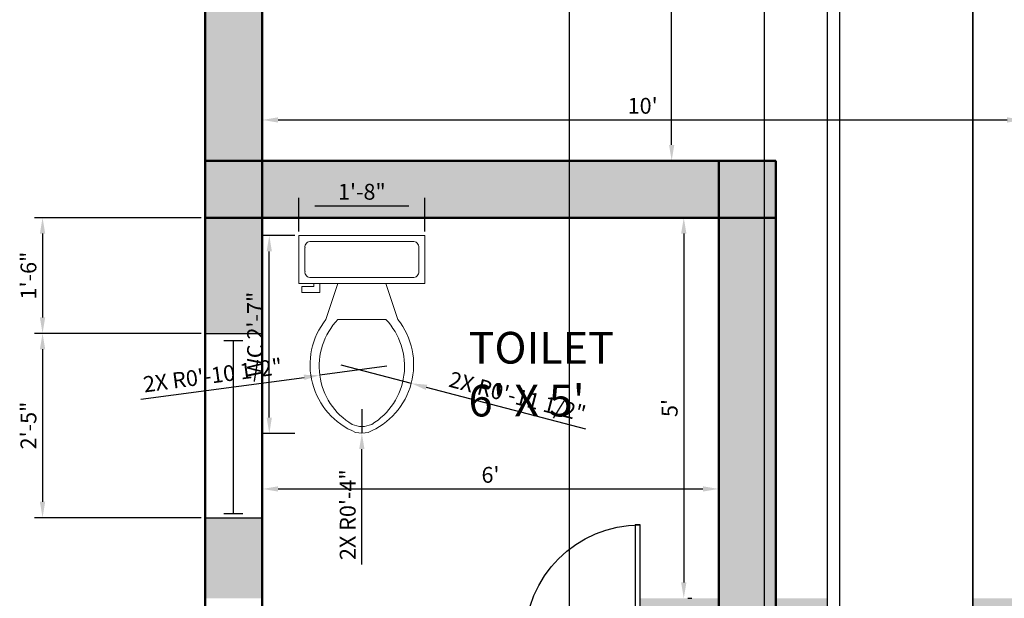
# Model space of a CAD drawing. Units: millimetres. Extents: x 2877 to 3173, y 802 to 1374.
# Tile 3 of 5: x 2879 to 3035, y 1144 to 1236. Entities that reach past the tile are written whole.
import ezdxf

# ---------------------------------------------------------------- set-up
doc = ezdxf.new("R2010")
doc.units = ezdxf.units.MM
for name, color, linetype, lineweight in [('A-AREA-IDEN', 150, 'Continuous', 25), ('A-FLOR-FIXT', 70, 'Continuous', 18), ('A-WALL-PATT', 3, 'Continuous', 13), ('dimensions', 140, 'Continuous', 18), ('doors', 10, 'Continuous', 25), ('walls', 50, 'Continuous', 50), ('windows', 190, 'Continuous', 25)]:
    doc.layers.add(name, color=color, linetype=linetype, lineweight=lineweight)
doc.styles.get("Standard").update_dxf_attribs({"font": 'arial.ttf'})
doc.dimstyles.new('ISO-25', dxfattribs={"dimtxt": 2.5, "dimasz": 2.5, "dimexe": 1.25, "dimexo": 0.625, "dimtad": 1, "dimdec": 0, "dimlunit": 3, "dimtxsty": 'Standard', "dimcen": 2.5, "dimadec": 0, "dimazin": 0, "dimtfac": 1, "dimtdec": 0, "dimtmove": 0, "dimatfit": 3, "dimfxl": 1, "dimarcsym": 0})

# ---------------------------------------------------------------- blocks, each defined once
blk = doc.blocks.new('*U2')
for p, q in [((0, 0), (0, -6)), ((40, 0), (40, -6))]:
    blk.add_line(p, q)
blk.add_lwpolyline([(0, 0), (0, 40), (1.75, 40), (1.75, 0)], close=True)
blk.add_arc((0, 0), 40, 0, 90)
blk = doc.blocks.new('Toilet - top')
for p, q in [((9.5, -6), (9.5, -2)), ((-8, -8.5), (-8, -8)), ((-7, -8), (-7, -9.5)), ((-4, -8), (-6, -14)), ((4, -8), (6, -14)), ((-10, -8.5), (-8, -8.5)), ((-10, -9.5), (-10, -8.5)), ((-7, -9.5), (-10, -9.5)), ((4, -14), (-4, -14))]:
    blk.add_line(p, q)
blk.add_lwpolyline([(10.5, -8), (10.5, 0), (-10.5, 0), (-10.5, -8)], close=True)
for points in [[(8.5, -1), (-8.5, -1)], [(-9.5, -2), (-9.5, -6)], [(-8.5, -7), (8.5, -7)]]:
    blk.add_lwpolyline(points)
for centre, radius, start, end in [((-8.62, -1.88), 0.884, 81.8699, 188.1301), ((8.62, -1.88), 0.884, 351.8699, 98.1301), ((-8.62, -6.12), 0.884, 171.8699, 278.1301), ((8.62, -6.12), 0.884, 261.8699, 8.1301), ((3.52, -21.58), 12.17, 141.4691, 247.9714), ((4.2, -21.82), 11.33, 136.3677, 238.9468), ((-3.52, -21.58), 12.17, 292.0284, 38.5307), ((-4.2, -21.82), 11.33, 301.053, 43.6321), ((0, -27.88), 4, 245.7318, 294.2682), ((0, -29), 4, 254.8605, 285.1395)]:
    blk.add_arc(centre, radius, start, end)
blk = doc.blocks.new('*U9')
for p, q in [((0, 4), (0, 0)), ((36, 4), (36, 0)), ((0, 2), (36, 2))]:
    blk.add_line(p, q)
blk = doc.blocks.new('*D10')
at = {"layer": 'Defpoints', "color": 0, "transparency": 16777216}
for p in [(3037.62, 1219.71), (2917.62, 1213.28), (3037.62, 1213.28)]:
    blk.add_point(p, dxfattribs=at)
at = {"layer": 'dimensions', "color": 0, "lineweight": -2, "transparency": 16777216}
for p, q in [((2917.62, 1213.9), (2917.62, 1220.96)), ((3037.62, 1213.9), (3037.62, 1220.96)), ((2920.12, 1219.71), (3035.12, 1219.71))]:
    blk.add_line(p, q, dxfattribs=at)
at = {"layer": 'dimensions', "color": 0, "transparency": 16777216}
for points in [[(2920.12, 1220.13), (2920.12, 1219.3), (2917.62, 1219.71)], [(3035.12, 1220.13), (3035.12, 1219.3), (3037.62, 1219.71)]]:
    blk.add_solid(points, dxfattribs=at)
at = {"layer": 'dimensions', "color": 0, "transparency": 16777216, "insert": (2977.62, 1221.62), "char_height": 2.5, "attachment_point": 5}
blk.add_mtext("10'", dxfattribs=at)
blk = doc.blocks.new('*D11')
at = {"layer": 'Defpoints', "color": 0, "transparency": 16777216}
for p in [(2982.2, 1333.28), (2982.2, 1333.28), (2982.2, 1213.28)]:
    blk.add_point(p, dxfattribs=at)
at = {"layer": 'dimensions', "color": 0, "lineweight": -2, "transparency": 16777216}
for p, q in [((2982.83, 1333.28), (2983.45, 1333.28)), ((2982.2, 1215.78), (2982.2, 1330.78)), ((2982.83, 1213.28), (2983.45, 1213.28))]:
    blk.add_line(p, q, dxfattribs=at)
at = {"layer": 'dimensions', "color": 0, "transparency": 16777216}
for points in [[(2981.79, 1330.78), (2982.62, 1330.78), (2982.2, 1333.28)], [(2981.79, 1215.78), (2982.62, 1215.78), (2982.2, 1213.28)]]:
    blk.add_solid(points, dxfattribs=at)
at = {"layer": 'dimensions', "color": 0, "transparency": 16777216, "insert": (2980.3, 1273.28), "char_height": 2.5, "attachment_point": 5, "rotation": 90}
blk.add_mtext("10'", dxfattribs=at)
blk = doc.blocks.new('*D16')
at = {"layer": 'Defpoints', "color": 0, "transparency": 16777216}
for p in [(2984.11, 1204.28), (2984.11, 1144.28), (2984.11, 1144.28)]:
    blk.add_point(p, dxfattribs=at)
at = {"layer": 'dimensions', "color": 0, "lineweight": -2, "transparency": 16777216}
for p, q in [((2984.74, 1204.28), (2985.36, 1204.28)), ((2984.11, 1201.78), (2984.11, 1146.78)), ((2984.74, 1144.28), (2985.36, 1144.28))]:
    blk.add_line(p, q, dxfattribs=at)
at = {"layer": 'dimensions', "color": 0, "transparency": 16777216}
for points in [[(2983.69, 1201.78), (2984.53, 1201.78), (2984.11, 1204.28)], [(2983.69, 1146.78), (2984.53, 1146.78), (2984.11, 1144.28)]]:
    blk.add_solid(points, dxfattribs=at)
at = {"layer": 'dimensions', "color": 0, "transparency": 16777216, "insert": (2982.21, 1174.28), "char_height": 2.5, "attachment_point": 5, "rotation": 90}
blk.add_mtext("5'", dxfattribs=at)
blk = doc.blocks.new('*D17')
at = {"layer": 'Defpoints', "color": 0, "transparency": 16777216}
for p in [(2989.62, 1161.52), (2917.62, 1160), (2989.62, 1160)]:
    blk.add_point(p, dxfattribs=at)
at = {"layer": 'dimensions', "color": 0, "lineweight": -2, "transparency": 16777216}
for p, q in [((2917.62, 1160.63), (2917.62, 1162.77)), ((2989.62, 1160.63), (2989.62, 1162.77)), ((2920.12, 1161.52), (2987.12, 1161.52))]:
    blk.add_line(p, q, dxfattribs=at)
at = {"layer": 'dimensions', "color": 0, "transparency": 16777216}
for points in [[(2920.12, 1161.94), (2920.12, 1161.11), (2917.62, 1161.52)], [(2987.12, 1161.94), (2987.12, 1161.11), (2989.62, 1161.52)]]:
    blk.add_solid(points, dxfattribs=at)
at = {"layer": 'dimensions', "color": 0, "transparency": 16777216, "insert": (2953.62, 1163.42), "char_height": 2.5, "attachment_point": 5}
blk.add_mtext("6'", dxfattribs=at)
blk = doc.blocks.new('*D26')
at = {"layer": 'Defpoints', "color": 0, "transparency": 16777216}
for p in [(2918.73, 1201.48), (2923.41, 1201.48), (2923.41, 1170.27)]:
    blk.add_point(p, dxfattribs=at)
at = {"layer": 'dimensions', "color": 0, "lineweight": -2, "transparency": 16777216}
for p, q in [((2922.78, 1201.48), (2917.48, 1201.48)), ((2918.73, 1172.77), (2918.73, 1198.98)), ((2922.78, 1170.27), (2917.48, 1170.27))]:
    blk.add_line(p, q, dxfattribs=at)
at = {"layer": 'dimensions', "color": 0, "transparency": 16777216}
for points in [[(2918.31, 1198.98), (2919.14, 1198.98), (2918.73, 1201.48)], [(2918.31, 1172.77), (2919.14, 1172.77), (2918.73, 1170.27)]]:
    blk.add_solid(points, dxfattribs=at)
at = {"layer": 'dimensions', "color": 0, "transparency": 16777216, "insert": (2916.81, 1185.88), "char_height": 2.5, "attachment_point": 5, "rotation": 90}
blk.add_mtext('WC 2\'-7"', dxfattribs=at)
blk = doc.blocks.new('*D27')
at = {"layer": 'Defpoints', "color": 0, "transparency": 16777216}
for p in [(2943.24, 1206.16), (2923.41, 1201.48), (2943.24, 1201.48)]:
    blk.add_point(p, dxfattribs=at)
at = {"layer": 'dimensions', "color": 0, "lineweight": -2, "transparency": 16777216}
for p, q in [((2923.41, 1202.11), (2923.41, 1207.41)), ((2943.24, 1202.11), (2943.24, 1207.41)), ((2925.91, 1206.16), (2940.74, 1206.16))]:
    blk.add_line(p, q, dxfattribs=at)
at = {"layer": 'dimensions', "color": 0, "transparency": 16777216}
for points in [[(2925.91, 1206.58), (2925.91, 1205.75), (2923.41, 1206.16)], [(2940.74, 1206.58), (2940.74, 1205.75), (2943.24, 1206.16)]]:
    blk.add_solid(points, dxfattribs=at)
at = {"layer": 'dimensions', "color": 0, "transparency": 16777216, "insert": (2933.33, 1208.06), "char_height": 2.5, "attachment_point": 5}
blk.add_mtext('1\'-8"', dxfattribs=at)
blk = doc.blocks.new('*D36')
at = {"layer": 'Defpoints', "color": 0, "transparency": 16777216}
for p in [(2908.62, 1301.43), (2917.62, 1301.43), (2917.62, 803.61)]:
    blk.add_point(p, dxfattribs=at)
at = {"layer": 'dimensions', "color": 0, "lineweight": -2, "transparency": 16777216}
for p, q in [((2908.62, 1300.81), (2908.62, 802.36)), ((2917.62, 1300.81), (2917.62, 802.36)), ((2911.12, 803.61), (2915.12, 803.61))]:
    blk.add_line(p, q, dxfattribs=at)
at = {"layer": 'dimensions', "color": 0, "transparency": 16777216}
for points in [[(2911.12, 804.03), (2911.12, 803.2), (2908.62, 803.61)], [(2915.12, 804.03), (2915.12, 803.2), (2917.62, 803.61)]]:
    blk.add_solid(points, dxfattribs=at)
at = {"layer": 'dimensions', "color": 0, "transparency": 16777216, "insert": (2913.12, 805.52), "char_height": 2.5, "attachment_point": 5}
blk.add_mtext('0\'-9"', dxfattribs=at)
blk = doc.blocks.new('*D44')
at = {"layer": 'Defpoints', "color": 0, "transparency": 16777216}
for p in [(2996.81, 1237.82), (3029.69, 1237.82), (3029.69, 803.61)]:
    blk.add_point(p, dxfattribs=at)
at = {"layer": 'dimensions', "color": 0, "lineweight": -2, "transparency": 16777216}
for p, q in [((2996.81, 1237.19), (2996.81, 802.36)), ((3029.69, 1237.19), (3029.69, 802.36)), ((2999.31, 803.61), (3027.19, 803.61))]:
    blk.add_line(p, q, dxfattribs=at)
at = {"layer": 'dimensions', "color": 0, "transparency": 16777216}
for points in [[(2999.31, 804.03), (2999.31, 803.2), (2996.81, 803.61)], [(3027.19, 804.03), (3027.19, 803.2), (3029.69, 803.61)]]:
    blk.add_solid(points, dxfattribs=at)
at = {"layer": 'dimensions', "color": 0, "transparency": 16777216, "insert": (3013.25, 805.52), "char_height": 2.5, "attachment_point": 5}
blk.add_mtext('2\'-9"', dxfattribs=at)
blk = doc.blocks.new('*D48')
at = {"layer": 'Defpoints', "color": 0, "transparency": 16777216}
for p in [(3029.73, 1367.94), (3006.77, 1144.28), (3029.73, 1144.28)]:
    blk.add_point(p, dxfattribs=at)
at = {"layer": 'dimensions', "color": 0, "lineweight": -2, "transparency": 16777216}
for p, q in [((3006.77, 1144.9), (3006.77, 1369.19)), ((3029.73, 1144.9), (3029.73, 1369.19)), ((3009.27, 1367.94), (3027.23, 1367.94))]:
    blk.add_line(p, q, dxfattribs=at)
at = {"layer": 'dimensions', "color": 0, "transparency": 16777216}
for points in [[(3009.27, 1368.36), (3009.27, 1367.52), (3006.77, 1367.94)], [(3027.23, 1368.36), (3027.23, 1367.52), (3029.73, 1367.94)]]:
    blk.add_solid(points, dxfattribs=at)
at = {"layer": 'dimensions', "color": 0, "transparency": 16777216, "insert": (3018.25, 1369.82), "char_height": 2.5, "attachment_point": 5}
blk.add_mtext('1\'-11"', dxfattribs=at)
blk = doc.blocks.new('*D49')
at = {"layer": 'Defpoints', "color": 0, "transparency": 16777216}
for p in [(3046.62, 1367.94), (3029.73, 1144.28), (3046.62, 1144.28)]:
    blk.add_point(p, dxfattribs=at)
at = {"layer": 'dimensions', "color": 0, "lineweight": -2, "transparency": 16777216}
for p, q in [((3029.73, 1144.9), (3029.73, 1369.19)), ((3046.62, 1144.9), (3046.62, 1369.19)), ((3032.23, 1367.94), (3044.12, 1367.94))]:
    blk.add_line(p, q, dxfattribs=at)
at = {"layer": 'dimensions', "color": 0, "transparency": 16777216}
for points in [[(3032.23, 1368.36), (3032.23, 1367.52), (3029.73, 1367.94)], [(3044.12, 1368.36), (3044.12, 1367.52), (3046.62, 1367.94)]]:
    blk.add_solid(points, dxfattribs=at)
at = {"layer": 'dimensions', "color": 0, "transparency": 16777216, "insert": (3038.18, 1369.84), "char_height": 2.5, "attachment_point": 5}
blk.add_mtext('1\'-5"', dxfattribs=at)
blk = doc.blocks.new('*D54')
at = {"layer": 'Defpoints', "color": 0, "transparency": 16777216}
for p in [(2908.62, 1204.28), (2882.96, 1186.06), (2908.62, 1186.06)]:
    blk.add_point(p, dxfattribs=at)
at = {"layer": 'dimensions', "color": 0, "lineweight": -2, "transparency": 16777216}
for p, q in [((2908, 1204.28), (2881.71, 1204.28)), ((2882.96, 1201.78), (2882.96, 1188.56)), ((2908, 1186.06), (2881.71, 1186.06))]:
    blk.add_line(p, q, dxfattribs=at)
at = {"layer": 'dimensions', "color": 0, "transparency": 16777216}
for points in [[(2882.54, 1201.78), (2883.38, 1201.78), (2882.96, 1204.28)], [(2882.54, 1188.56), (2883.38, 1188.56), (2882.96, 1186.06)]]:
    blk.add_solid(points, dxfattribs=at)
at = {"layer": 'dimensions', "color": 0, "transparency": 16777216, "insert": (2881.06, 1195.17), "char_height": 2.5, "attachment_point": 5, "rotation": 90}
blk.add_mtext('1\'-6"', dxfattribs=at)
blk = doc.blocks.new('*D55')
at = {"layer": 'Defpoints', "color": 0, "transparency": 16777216}
for p in [(2908.62, 1186.06), (2882.96, 1156.99), (2908.62, 1156.99)]:
    blk.add_point(p, dxfattribs=at)
at = {"layer": 'dimensions', "color": 0, "lineweight": -2, "transparency": 16777216}
for p, q in [((2908, 1186.06), (2881.71, 1186.06)), ((2882.96, 1183.56), (2882.96, 1159.49)), ((2908, 1156.99), (2881.71, 1156.99))]:
    blk.add_line(p, q, dxfattribs=at)
at = {"layer": 'dimensions', "color": 0, "transparency": 16777216}
for points in [[(2882.54, 1183.56), (2883.38, 1183.56), (2882.96, 1186.06)], [(2882.54, 1159.49), (2883.38, 1159.49), (2882.96, 1156.99)]]:
    blk.add_solid(points, dxfattribs=at)
at = {"layer": 'dimensions', "color": 0, "transparency": 16777216, "insert": (2881.06, 1171.52), "char_height": 2.5, "attachment_point": 5, "rotation": 90}
blk.add_mtext('2\'-5"', dxfattribs=at)
blk = doc.blocks.new('*D58')
at = {"layer": 'Defpoints', "color": 0, "transparency": 16777216}
for p in [(2966.07, 1367.94), (2908.62, 943.28), (2966.07, 943.28)]:
    blk.add_point(p, dxfattribs=at)
at = {"layer": 'dimensions', "color": 0, "lineweight": -2, "transparency": 16777216}
for p, q in [((2908.62, 943.9), (2908.62, 1369.19)), ((2966.07, 943.9), (2966.07, 1369.19)), ((2911.12, 1367.94), (2963.57, 1367.94))]:
    blk.add_line(p, q, dxfattribs=at)
at = {"layer": 'dimensions', "color": 0, "transparency": 16777216}
for points in [[(2911.12, 1368.36), (2911.12, 1367.52), (2908.62, 1367.94)], [(2963.57, 1368.36), (2963.57, 1367.52), (2966.07, 1367.94)]]:
    blk.add_solid(points, dxfattribs=at)
at = {"layer": 'dimensions', "color": 0, "transparency": 16777216, "insert": (2937.34, 1369.86), "char_height": 2.5, "attachment_point": 5}
blk.add_mtext('4\'-9 1/2"', dxfattribs=at)
blk = doc.blocks.new('*D59')
at = {"layer": 'Defpoints', "color": 0, "transparency": 16777216}
for p in [(3008.74, 1367.94), (2966.07, 943.28), (3008.74, 943.28)]:
    blk.add_point(p, dxfattribs=at)
at = {"layer": 'dimensions', "color": 0, "lineweight": -2, "transparency": 16777216}
for p, q in [((2966.07, 943.9), (2966.07, 1369.19)), ((3008.74, 943.9), (3008.74, 1369.19)), ((2968.57, 1367.94), (3006.24, 1367.94))]:
    blk.add_line(p, q, dxfattribs=at)
at = {"layer": 'dimensions', "color": 0, "transparency": 16777216}
for points in [[(2968.57, 1368.36), (2968.57, 1367.52), (2966.07, 1367.94)], [(3006.24, 1368.36), (3006.24, 1367.52), (3008.74, 1367.94)]]:
    blk.add_solid(points, dxfattribs=at)
at = {"layer": 'dimensions', "color": 0, "transparency": 16777216, "insert": (2987.4, 1369.86), "char_height": 2.5, "attachment_point": 5}
blk.add_mtext('3\'-6 1/2"', dxfattribs=at)
blk = doc.blocks.new('*D66')
at = {"layer": 'Defpoints', "color": 0, "transparency": 16777216}
for p in [(2917.62, 1257.52), (2996.81, 1237.82), (2996.81, 803.61)]:
    blk.add_point(p, dxfattribs=at)
at = {"layer": 'dimensions', "color": 0, "lineweight": -2, "transparency": 16777216}
for p, q in [((2917.62, 1256.89), (2917.62, 802.36)), ((2996.81, 1237.19), (2996.81, 802.36)), ((2920.12, 803.61), (2994.31, 803.61))]:
    blk.add_line(p, q, dxfattribs=at)
at = {"layer": 'dimensions', "color": 0, "transparency": 16777216}
for points in [[(2920.12, 804.03), (2920.12, 803.2), (2917.62, 803.61)], [(2994.31, 804.03), (2994.31, 803.2), (2996.81, 803.61)]]:
    blk.add_solid(points, dxfattribs=at)
at = {"layer": 'dimensions', "color": 0, "transparency": 16777216, "insert": (2957.22, 805.52), "char_height": 2.5, "attachment_point": 5}
blk.add_mtext('6\'-7"', dxfattribs=at)
blk = doc.blocks.new('*D72')
at = {"layer": 'Defpoints', "color": 0, "transparency": 16777216}
for p in [(2930, 1181.1), (2941.12, 1178.18)]:
    blk.add_point(p, dxfattribs=at)
at = {"layer": 'dimensions', "color": 0, "lineweight": -2, "transparency": 16777216}
for p, q in [((2930, 1181.1), (2941.12, 1178.18)), ((2968.65, 1170.95), (2943.54, 1177.54))]:
    blk.add_line(p, q, dxfattribs=at)
at = {"layer": 'dimensions', "color": 0, "transparency": 16777216}
blk.add_solid([(2943.64, 1177.95), (2943.43, 1177.14), (2941.12, 1178.18)], dxfattribs=at)
at = {"layer": 'dimensions', "color": 0, "transparency": 16777216, "insert": (2957.79, 1175.78), "char_height": 2.5, "attachment_point": 5, "rotation": 345.2815}
blk.add_mtext('2X R0\'-11 1/2"', dxfattribs=at)
blk = doc.blocks.new('*D73')
at = {"layer": 'Defpoints', "color": 0, "transparency": 16777216}
for p in [(2937.29, 1180.88), (2926.69, 1179.45)]:
    blk.add_point(p, dxfattribs=at)
at = {"layer": 'dimensions', "color": 0, "lineweight": -2, "transparency": 16777216}
for p, q in [((2937.29, 1180.88), (2926.69, 1179.45)), ((2898.47, 1175.66), (2924.21, 1179.12))]:
    blk.add_line(p, q, dxfattribs=at)
at = {"layer": 'dimensions', "color": 0, "transparency": 16777216}
blk.add_solid([(2924.16, 1179.53), (2924.27, 1178.71), (2926.69, 1179.45)], dxfattribs=at)
at = {"layer": 'dimensions', "color": 0, "transparency": 16777216, "insert": (2909.85, 1179.12), "char_height": 2.5, "attachment_point": 5, "rotation": 7.6546}
blk.add_mtext('2X R0\'-10 1/2"', dxfattribs=at)
blk = doc.blocks.new('*D74')
at = {"layer": 'Defpoints', "color": 0, "transparency": 16777216}
for p in [(2933.33, 1174.09), (2933.33, 1170.32)]:
    blk.add_point(p, dxfattribs=at)
at = {"layer": 'dimensions', "color": 0, "lineweight": -2, "transparency": 16777216}
for p, q in [((2933.33, 1174.09), (2933.33, 1170.32)), ((2933.33, 1149.61), (2933.33, 1167.82))]:
    blk.add_line(p, q, dxfattribs=at)
at = {"layer": 'dimensions', "color": 0, "transparency": 16777216}
blk.add_solid([(2932.91, 1167.82), (2933.74, 1167.82), (2933.33, 1170.32)], dxfattribs=at)
at = {"layer": 'dimensions', "color": 0, "transparency": 16777216, "insert": (2931.42, 1157.46), "char_height": 2.5, "attachment_point": 5, "rotation": 89.9983}
blk.add_mtext('2X R0\'-4"', dxfattribs=at)

msp = doc.modelspace()

# ---------------------------------------------------------------- hatches: boundary and pattern name
at = {"layer": 'A-WALL-PATT'}
h = msp.add_hatch(color=256, dxfattribs=at)
h.dxf.hatch_style = 1
h.paths.add_polyline_path([(3046.62, 1333.28), (3037.62, 1333.28), (3037.62, 1273.28), (3046.62, 1273.28)])
h.paths.add_polyline_path([(3046.62, 1273.28), (3037.62, 1273.28), (3037.62, 1264.28), (3046.62, 1264.28)])
h.paths.add_polyline_path([(3046.62, 1264.28), (3037.62, 1264.28), (3037.62, 1204.28), (3046.62, 1204.28)])
h.paths.add_polyline_path([(3136.62, 1273.28), (3099.39, 1273.28), (3099.39, 1264.28), (3136.62, 1264.28)])
h.paths.add_polyline_path([(3145.62, 1273.28), (3136.62, 1273.28), (3136.62, 1264.28), (3145.62, 1264.28)])
h.paths.add_polyline_path([(3145.62, 1264.28), (3136.62, 1264.28), (3136.62, 1198.76), (3145.62, 1198.76)])
h.paths.add_polyline_path([(3145.62, 1333.28), (3136.62, 1333.28), (3136.62, 1273.28), (3145.62, 1273.28)])
h.paths.add_polyline_path([(3145.62, 1342.28), (3136.62, 1342.28), (3136.62, 1333.28), (3145.62, 1333.28)])
h.paths.add_polyline_path([(3136.62, 1342.28), (3046.62, 1342.28), (3046.62, 1333.28), (3136.62, 1333.28)])
h.paths.add_polyline_path([(3046.62, 1342.28), (3037.62, 1342.28), (3037.62, 1333.28), (3046.62, 1333.28)])
h.paths.add_polyline_path([(2917.62, 1333.28), (2908.62, 1333.28), (2908.62, 1301.43), (2917.62, 1301.43)])
h.paths.add_polyline_path([(2917.62, 1257.52), (2908.62, 1257.52), (2908.62, 1213.28), (2917.62, 1213.28)])
h.paths.add_polyline_path([(2989.62, 1213.28), (2917.62, 1213.28), (2917.62, 1204.28), (2989.62, 1204.28)])
h.paths.add_polyline_path([(2998.62, 1213.28), (2989.62, 1213.28), (2989.62, 1204.28), (2998.62, 1204.28)])
h.paths.add_polyline_path([(2998.62, 1204.28), (2989.62, 1204.28), (2989.62, 1144.28), (2998.62, 1144.28)])
h.paths.add_polyline_path([(2998.62, 1144.28), (2989.62, 1144.28), (2989.62, 1135.28), (2998.62, 1135.28)])
h.paths.add_polyline_path([(2989.62, 1144.28), (2977.25, 1144.28), (2977.25, 1137.64), (2977.25, 1135.28), (2989.62, 1135.28)])
h.paths.add_polyline_path([(3006.77, 1141.79), (3006.77, 1144.28), (2998.62, 1144.28), (2998.62, 1135.28), (3007.71, 1135.28, -0.072018)])
h.paths.add_polyline_path([(3046.62, 1135.28), (3037.62, 1135.28), (3037.62, 1012.28), (3046.62, 1012.28)])
h.paths.add_polyline_path([(3046.62, 1144.28), (3037.62, 1144.28), (3037.62, 1135.28), (3046.62, 1135.28)])
h.paths.add_polyline_path([(3037.62, 1144.28), (3029.73, 1144.28), (3029.73, 1141.79), (3029.73, 1135.28), (3037.62, 1135.28)])
h.paths.add_polyline_path([(3145.62, 1158.87), (3136.62, 1158.87), (3136.62, 1012.28), (3145.62, 1012.28)])
h.paths.add_polyline_path([(3145.62, 1003.28), (3136.62, 1003.28), (3136.62, 838.28), (3145.62, 838.28)])
h.paths.add_polyline_path([(3145.62, 1012.28), (3136.62, 1012.28), (3136.62, 1003.28), (3145.62, 1003.28)])
h.paths.add_polyline_path([(3136.62, 1012.28), (3109.83, 1012.28), (3109.83, 1006.01), (3109.83, 1003.28), (3136.62, 1003.28)])
h.paths.add_polyline_path([(3073.41, 1012.28), (3046.62, 1012.28), (3046.62, 1003.28), (3073.41, 1003.28), (3073.41, 1006.01)])
h.paths.add_polyline_path([(3046.62, 1012.28), (3037.62, 1012.28), (3037.62, 1003.28), (3046.62, 1003.28)])
h.paths.add_polyline_path([(3046.62, 1003.28), (3037.62, 1003.28), (3037.62, 943.28), (3046.62, 943.28)])
h.paths.add_polyline_path([(3136.62, 838.28), (2917.62, 838.28), (2917.62, 829.28), (3136.62, 829.28)])
h.paths.add_polyline_path([(3145.62, 838.28), (3136.62, 838.28), (3136.62, 829.28), (3145.62, 829.28)])
h.paths.add_polyline_path([(2917.62, 934.28), (2908.62, 934.28), (2908.62, 838.28), (2917.62, 838.28)])
h.paths.add_polyline_path([(2917.62, 838.28), (2908.62, 838.28), (2908.62, 829.28), (2917.62, 829.28)])
h.paths.add_polyline_path([(2917.62, 943.28), (2908.62, 943.28), (2908.62, 934.28), (2917.62, 934.28)])
h.paths.add_polyline_path([(2966.07, 943.28), (2917.62, 943.28), (2917.62, 934.28), (2966.07, 934.28)])
h.paths.add_polyline_path([(3046.62, 943.28), (3037.62, 943.28), (3037.62, 934.28), (3046.62, 934.28)])
h.paths.add_polyline_path([(3037.62, 943.28), (3008.74, 943.28), (3008.74, 934.28), (3037.62, 934.28)])
h = msp.add_hatch(color=256, dxfattribs=at)
h.dxf.hatch_style = 1
h.paths.add_polyline_path([(2917.62, 1213.28), (2908.62, 1213.28), (2908.62, 1204.28), (2917.62, 1204.28)])
h = msp.add_hatch(color=256, dxfattribs=at)
h.dxf.hatch_style = 1
h.paths.add_polyline_path([(2917.62, 1204.28), (2908.62, 1204.28), (2908.62, 1186.06), (2917.62, 1186.06)])
h.paths.add_polyline_path([(2917.62, 1156.99), (2908.62, 1156.99), (2908.62, 1144.28), (2917.62, 1144.28)])

# ---------------------------------------------------------------- linework, layer by layer
at = {"layer": 'walls'}
for p, q in [((2908.62, 1342.28), (2908.62, 829.28)), ((2917.62, 1342.28), (2917.62, 829.28)), ((2908.62, 1213.28), (2998.62, 1213.28)), ((2989.62, 1213.28), (2989.62, 1135.28)), ((2998.62, 1213.28), (2998.62, 1135.28)), ((2908.62, 1204.28), (2998.62, 1204.28))]:
    msp.add_line(p, q, dxfattribs=at)
at = {"layer": 'windows'}
for p, q in [((2908.62, 1186.06), (2917.62, 1186.06)), ((2908.62, 1156.99), (2917.62, 1156.99))]:
    msp.add_line(p, q, dxfattribs=at)

# ---------------------------------------------------------------- block references
at = {"layer": 'A-FLOR-FIXT', "xscale": 0.9444251569504508, "yscale": 0.9444251569504508, "zscale": 0.9444251569504508}
msp.add_blockref('Toilet - top', (2933.33, 1201.48), dxfattribs=at)
at = {"layer": 'doors', "xscale": -0.4552510015893225, "yscale": 0.4552510015893225, "zscale": 0.4552510015893225}
msp.add_blockref('*U2', (2977.25, 1137.64), dxfattribs=at)
at = {"layer": 'doors', "xscale": 0.5739608518723968, "yscale": 0.5739608518723968, "zscale": 0.5739608518723968, "rotation": 180}
msp.add_blockref('*U2', (3029.73, 1141.79), dxfattribs=at)
at = {"layer": 'windows', "xscale": 0.7577459519969472, "yscale": 0.7577459519969472, "zscale": 0.7577459519969472, "rotation": 90}
msp.add_blockref('*U9', (2914.58, 1157.67), dxfattribs=at)

# ---------------------------------------------------------------- texts
at = {"layer": 'A-AREA-IDEN', "insert": (2950.16, 1186.29), "char_height": 5, "attachment_point": 1}
msp.add_mtext_dynamic_manual_height_columns("TOILET\\P6' X 5'", width=32.1304, gutter_width=12.5, heights=[0], dxfattribs=at)

# ---------------------------------------------------------------- dimensions: what is measured, and where the dimension line sits
at = {"layer": 'dimensions'}
for base, p1, p2, override, picture, middle in [((2966.066, 1367.9388), (2908.6223, 943.2763), (2966.066, 943.2763), {"dimdec": 1, "dimlfac": 1, "dimrnd": 0, "dimzin": 1, "dimdsep": 46, "dimlunit": 4, "dimfrac": 2}, '*D58', (2937.3441, 1369.8564)), ((3008.74, 1367.94), (2966.07, 943.28), (3008.74, 943.28), {"dimdec": 1, "dimlfac": 1, "dimrnd": 0, "dimzin": 1, "dimdsep": 46, "dimlunit": 4, "dimfrac": 2}, '*D59', (2987.4, 1369.86)), ((3029.73, 1367.94), (3006.77, 1144.28), (3029.73, 1144.28), {"dimdec": 1, "dimlfac": 1, "dimrnd": 0, "dimzin": 1, "dimdsep": 46, "dimlunit": 4, "dimfrac": 2}, '*D48', (3018.25, 1369.82)), ((3046.62, 1367.94), (3029.73, 1144.28), (3046.62, 1144.28), {"dimdec": 1, "dimlfac": 1, "dimrnd": 0, "dimzin": 1, "dimdsep": 46, "dimlunit": 4, "dimfrac": 2}, '*D49', (3038.18, 1369.84)), ((2917.62, 803.61), (2908.62, 1301.43), (2917.62, 1301.43), {"dimdec": 1, "dimlfac": 1, "dimrnd": 0, "dimzin": 1, "dimdsep": 46, "dimlunit": 4, "dimfrac": 2}, '*D36', (2913.12, 805.52)), ((2996.81, 803.61), (2917.62, 1257.52), (2996.81, 1237.82), {"dimdec": 1, "dimlfac": 1, "dimrnd": 0, "dimzin": 1, "dimdsep": 46, "dimlunit": 4, "dimfrac": 2}, '*D66', (2957.22, 805.52)), ((3029.69, 803.61), (2996.81, 1237.82), (3029.69, 1237.82), {"dimdec": 1, "dimlfac": 1, "dimrnd": 0, "dimzin": 1, "dimdsep": 46, "dimlunit": 4, "dimfrac": 2}, '*D44', (3013.25, 805.52)), ((3037.62, 1219.71), (2917.62, 1213.28), (3037.62, 1213.28), {"dimclrd": 0, "dimclre": 0, "dimclrt": 0}, '*D10', (2977.62, 1221.62)), ((2943.24, 1206.16), (2923.41, 1201.48), (2943.24, 1201.48), {"dimdec": 1, "dimlfac": 1, "dimrnd": 0, "dimzin": 1, "dimdsep": 46, "dimlunit": 4, "dimfrac": 2}, '*D27', (2933.33, 1208.06)), ((2989.62, 1161.52), (2917.62, 1160), (2989.62, 1160), {"dimclrd": 0, "dimclre": 0, "dimclrt": 0}, '*D17', (2953.62, 1163.42))]:
    dim = msp.add_linear_dim(base=base, p1=p1, p2=p2, dimstyle='ISO-25', override=override, dxfattribs=at)
    dim.commit()
    dim.dimension.update_dxf_attribs({"geometry": picture, "text_midpoint": middle})
for base, p1, p2, override, picture, middle in [((2982.2, 1333.28), (2982.2, 1213.28), (2982.2, 1333.28), {"dimclrd": 0, "dimclre": 0, "dimclrt": 0}, '*D11', (2980.3, 1273.28)), ((2882.96, 1186.06), (2908.62, 1204.28), (2908.62, 1186.06), {"dimdec": 1, "dimlfac": 1, "dimrnd": 0, "dimzin": 1, "dimdsep": 46, "dimlunit": 4, "dimfrac": 2}, '*D54', (2881.06, 1195.17)), ((2984.11, 1144.28), (2984.11, 1204.28), (2984.11, 1144.28), {"dimclrd": 0, "dimclre": 0, "dimclrt": 0}, '*D16', (2982.21, 1174.28)), ((2882.96, 1156.99), (2908.62, 1186.06), (2908.62, 1156.99), {"dimdec": 1, "dimlfac": 1, "dimrnd": 0, "dimzin": 1, "dimdsep": 46, "dimlunit": 4, "dimfrac": 2}, '*D55', (2881.06, 1171.52))]:
    dim = msp.add_linear_dim(base=base, p1=p1, p2=p2, angle=90, dimstyle='ISO-25', override=override, dxfattribs=at)
    dim.commit()
    dim.dimension.update_dxf_attribs({"geometry": picture, "text_midpoint": middle})
dim = msp.add_linear_dim(base=(2918.73, 1201.48), p1=(2923.41, 1170.27), p2=(2923.41, 1201.48), angle=90, text='WC <>', dimstyle='ISO-25', override={"dimdec": 1, "dimlfac": 1, "dimrnd": 0, "dimzin": 1, "dimdsep": 46, "dimlunit": 4, "dimfrac": 2}, dxfattribs=at)
dim.commit()
dim.dimension.update_dxf_attribs({"geometry": '*D26', "text_midpoint": (2916.81, 1185.88)})
for center, mpoint, picture, middle in [((2937.29, 1180.88), (2926.69, 1179.45), '*D73', (2909.85, 1179.12)), ((2930, 1181.1), (2941.12, 1178.18), '*D72', (2957.79, 1175.78)), ((2933.33, 1174.09), (2933.33, 1170.32), '*D74', (2931.42, 1157.46))]:
    dim = msp.add_radius_dim(center=center, mpoint=mpoint, text='2X <>', dimstyle='ISO-25', override={"dimdec": 1, "dimlfac": 1, "dimrnd": 0, "dimzin": 1, "dimdsep": 46, "dimlunit": 4, "dimfrac": 2}, dxfattribs=at)
    dim.commit()
    dim.dimension.update_dxf_attribs({"geometry": picture, "text_midpoint": middle})

doc.saveas('drawing.dxf')
